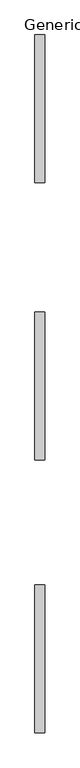
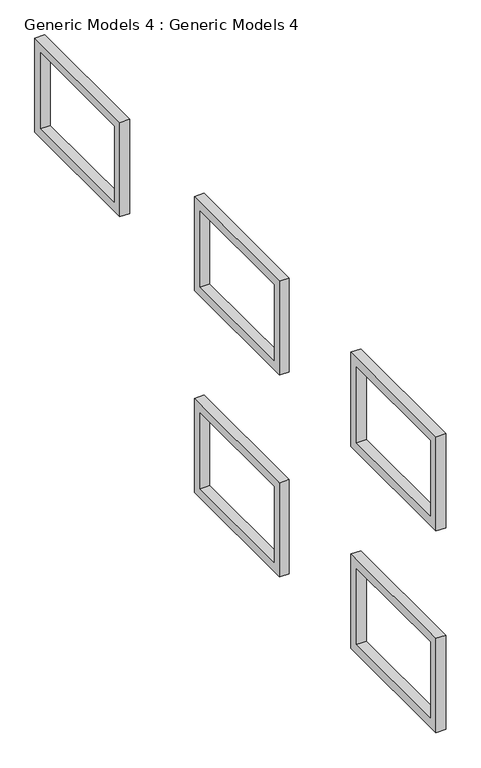
"""IFC4 building model written with IfcOpenShell, lengths in millimetres: proxy geometry, Generic Models 4 : Generic Models 4."""

from ifc_helpers import new_model, si_unit, frame, origin, place, context, project, spatial, polyline, outline, extrude, source, transform, mapped, element, save


def generic_models_4_generic_models_4_3a3d2180(model_context):
    return source(origin(), model_context, "Body", "SweptSolid", [
        extrude(outline(polyline([(504.6061648, 5765.2), (504.6061648, 4200.4), (-1810.1938352, 4200.4), (-1810.1938352, 5765.2), (504.6061648, 5765.2)]), holes=[polyline([(352.2061648, 5612.8), (-1657.7938352, 5612.8), (-1657.7938352, 4352.8), (352.2061648, 4352.8), (352.2061648, 5612.8)])]), frame((4139.9525369, 0.0, 0.0), z_axis=(1.0, 0.0, 0.0), x_axis=(0.0, 1.0, 0.0)), (0.0, 0.0, 1.0), 152.4),
        extrude(outline(polyline([(4771.8061648, 5765.2), (4771.8061648, 4200.4), (2457.0061648, 4200.4), (2457.0061648, 5765.2), (4771.8061648, 5765.2)]), holes=[polyline([(4619.4061648, 5612.8), (2609.4061648, 5612.8), (2609.4061648, 4352.8), (4619.4061648, 4352.8), (4619.4061648, 5612.8)])]), frame((4139.9525369, 0.0, 0.0), z_axis=(1.0, 0.0, 0.0), x_axis=(0.0, 1.0, 0.0)), (0.0, 0.0, 1.0), 152.4),
        extrude(outline(polyline([(9115.2061648, 5765.2), (9115.2061648, 4200.4), (6800.4061648, 4200.4), (6800.4061648, 5765.2), (9115.2061648, 5765.2)]), holes=[polyline([(8962.8061648, 5612.8), (6952.8061648, 5612.8), (6952.8061648, 4352.8), (8962.8061648, 4352.8), (8962.8061648, 5612.8)])]), frame((4139.9525369, 0.0, 0.0), z_axis=(1.0, 0.0, 0.0), x_axis=(0.0, 1.0, 0.0)), (0.0, 0.0, 1.0), 152.4),
        extrude(outline(polyline([(504.6061648, 2412.4), (504.6061648, 847.6), (-1810.1938352, 847.6), (-1810.1938352, 2412.4), (504.6061648, 2412.4)]), holes=[polyline([(352.2061648, 2260.0), (-1657.7938352, 2260.0), (-1657.7938352, 1000.0), (352.2061648, 1000.0), (352.2061648, 2260.0)])]), frame((4139.9525369, 0.0, 0.0), z_axis=(1.0, 0.0, 0.0), x_axis=(0.0, 1.0, 0.0)), (0.0, 0.0, 1.0), 152.4),
        extrude(outline(polyline([(4771.8061648, 2412.4), (4771.8061648, 847.6), (2457.0061648, 847.6), (2457.0061648, 2412.4), (4771.8061648, 2412.4)]), holes=[polyline([(4619.4061648, 2260.0), (2609.4061648, 2260.0), (2609.4061648, 1000.0), (4619.4061648, 1000.0), (4619.4061648, 2260.0)])]), frame((4139.9525369, 0.0, 0.0), z_axis=(1.0, 0.0, 0.0), x_axis=(0.0, 1.0, 0.0)), (0.0, 0.0, 1.0), 152.4),
    ])


if __name__ == "__main__":
    model = new_model("IFC4")
    model_context = context("Model", 3, world=origin())
    ifc_project = project(units=[si_unit("LENGTHUNIT", "METRE", prefix="MILLI")], contexts=[model_context])
    site = spatial("IfcSite", under=ifc_project)
    building = spatial("IfcBuilding", under=site)
    placement = place(None, origin())
    generic_models_4_generic_models_4_shape = generic_models_4_generic_models_4_3a3d2180(model_context)
    element("IfcBuildingElementProxy", 1, Name="Generic Models 4 : Generic Models 4", ObjectType="Generic Models 4 : Generic Models 4", at=placement, inside=building, context=model_context, shape_type="MappedRepresentation", body=[
        mapped(generic_models_4_generic_models_4_shape, transform((0.0, 0.0, 0.0), x_axis=(1.0, 0.0, 0.0), y_axis=(0.0, 1.0, 0.0), z_axis=(0.0, 0.0, 1.0))),
    ])
    save(model, "model.ifc")

# Revit data of these elements
# Element 1 (IfcBuildingElementProxy, "Generic Models 4 : Generic Models 4")
#   Materials on its faces: "WALL PAINT"
# Materials
#   "WALL PAINT": class "Generic", colour RGB 120 120 120, transparency 0, Cost = 0
